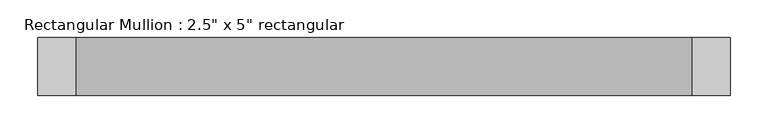
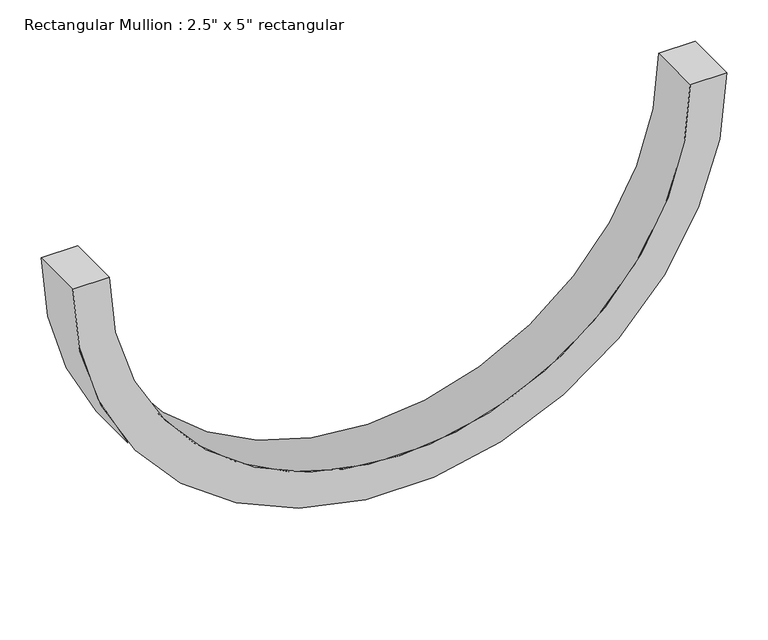
"""IFC4 building model written with IfcOpenShell, lengths in millimetres: member geometry."""

from ifc_helpers import new_model, si_unit, point, frame, frame_2d, origin, place, context, project, spatial, polyline, circle_curve, trimmed, segment, composite_curve, outline, extrude, source, transform, mapped, element, save


def member_fb5b44a5(model_context):
    return source(origin(), model_context, "Body", "SweptSolid", [
        extrude(outline(composite_curve([segment(trimmed(circle_curve(frame_2d((0.0, -457.2)), 457.2), [point((0.0, -914.4))], [point((0.0, 0.0))], False, "CARTESIAN"), True, "CONTINUOUS"), segment(polyline([(0.0, 0.0), (0.0, -50.8)]), True, "CONTINUOUS"), segment(trimmed(circle_curve(frame_2d((0.0, -457.2)), 406.4), [point((0.0, -50.8))], [point((0.0, -863.6))], True, "CARTESIAN"), True, "CONTINUOUS"), segment(polyline([(0.0, -863.6), (0.0, -914.4)]), True, "CONTINUOUS")], self_intersect=False)), frame((0.0, -38.1, 0.0), z_axis=(0.0, 1.0, 0.0), x_axis=(0.0, 0.0, 1.0)), (0.0, 0.0, 1.0), 76.2),
    ])


if __name__ == "__main__":
    model = new_model("IFC4")
    model_context = context("Model", 3, world=origin())
    ifc_project = project(units=[si_unit("LENGTHUNIT", "METRE", prefix="MILLI")], contexts=[model_context])
    site = spatial("IfcSite", under=ifc_project)
    building = spatial("IfcBuilding", under=site)
    placement = place(None, origin())
    member_shape = member_fb5b44a5(model_context)
    element("IfcMember", 1, ObjectType="Rectangular Mullion : 2.5\" x 5\" rectangular", at=placement, inside=building, context=model_context, shape_type="MappedRepresentation", body=[
        mapped(member_shape, transform((0.0, 0.0, 0.0), x_axis=(1.0, 0.0, 0.0), y_axis=(0.0, 1.0, 0.0), z_axis=(0.0, 0.0, 1.0))),
    ])
    save(model, "model.ifc")

# Revit data of these elements
# Type "Rectangular Mullion : 2.5\" x 5\" rectangular"
#   built-in parameter 1007304 = 0.25 (stored number, unit not read)
#   built-in parameter 1007301 = 0.0833333 (stored number, unit not read)
#   built-in parameter 1007300 = 0.0833333 (stored number, unit not read)
# Element 1 (IfcMember, "Rectangular Mullion : 2.5\" x 5\" rectangular")
#   Materials on its faces: "Aluminum"
# Materials
#   "Aluminum": class "Metal", colour RGB 244 245 246, transparency 0, Description = "Aluminum 6061", Cost = 0
